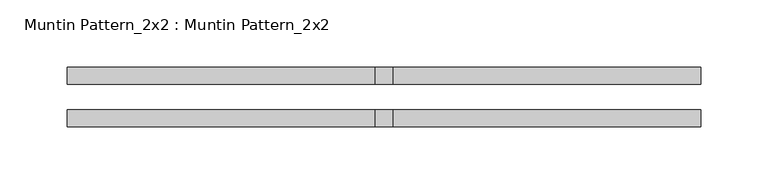
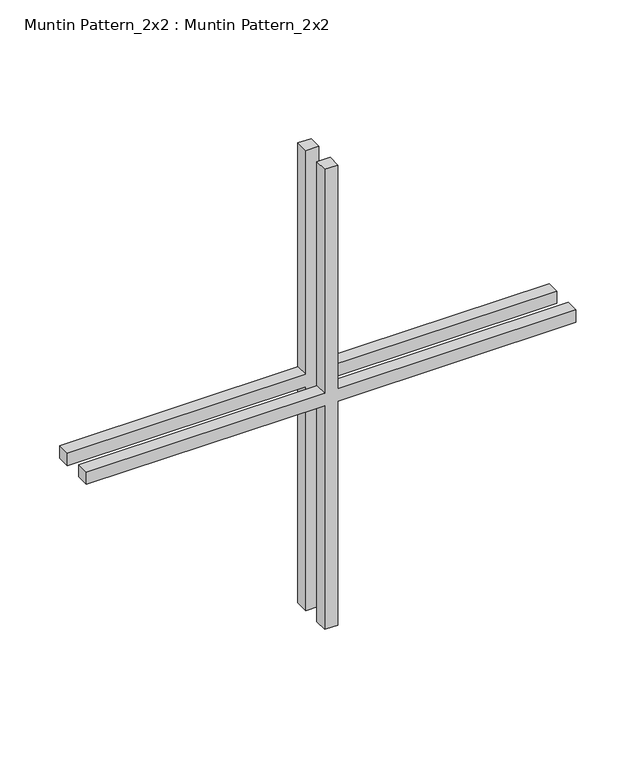
"""IFC4 building model written with IfcOpenShell, lengths in millimetres: proxy geometry, Muntin Pattern_2x2 : Muntin Pattern_2x2."""

from ifc_helpers import new_model, si_unit, frame, origin, place, context, project, spatial, polyline, outline, extrude, source, transform, mapped, element, save


def muntin_pattern_2x2_muntin_pattern_2x2_7d820091(model_context):
    return source(origin(), model_context, "Body", "SweptSolid", [
        extrude(outline(polyline([(241.3, -6.35), (241.3, -236.5375), (228.6, -236.5375), (228.6, -6.35), (0.0, -6.35), (0.0, 6.35), (228.6, 6.35), (228.6, 236.5375), (241.3, 236.5375), (241.3, 6.35), (469.9, 6.35), (469.9, -6.35), (241.3, -6.35)])), frame((0.0, 9.525, 0.0), z_axis=(0.0, 1.0, 0.0), x_axis=(0.0, 0.0, 1.0)), (0.0, 0.0, 1.0), 12.7),
        extrude(outline(polyline([(241.3, -6.35), (241.3, -236.5375), (228.6, -236.5375), (228.6, -6.35), (0.0, -6.35), (0.0, 6.35), (228.6, 6.35), (228.6, 236.5375), (241.3, 236.5375), (241.3, 6.35), (469.9, 6.35), (469.9, -6.35), (241.3, -6.35)])), frame((0.0, -22.225, 0.0), z_axis=(0.0, 1.0, 0.0), x_axis=(0.0, 0.0, 1.0)), (0.0, 0.0, 1.0), 12.7),
    ])


if __name__ == "__main__":
    model = new_model("IFC4")
    model_context = context("Model", 3, world=origin())
    ifc_project = project(units=[si_unit("LENGTHUNIT", "METRE", prefix="MILLI")], contexts=[model_context])
    site = spatial("IfcSite", under=ifc_project)
    building = spatial("IfcBuilding", under=site)
    placement = place(None, origin())
    muntin_pattern_2x2_muntin_pattern_2x2_shape = muntin_pattern_2x2_muntin_pattern_2x2_7d820091(model_context)
    element("IfcBuildingElementProxy", 1, Name="Muntin Pattern_2x2 : Muntin Pattern_2x2", ObjectType="Muntin Pattern_2x2 : Muntin Pattern_2x2", at=placement, inside=building, context=model_context, shape_type="MappedRepresentation", body=[
        mapped(muntin_pattern_2x2_muntin_pattern_2x2_shape, transform((0.0, 0.0, 0.0), x_axis=(1.0, 0.0, 0.0), y_axis=(0.0, 1.0, 0.0), z_axis=(0.0, 0.0, 1.0))),
    ])
    save(model, "model.ifc")

# Revit data of these elements
# Type "Muntin Pattern_2x2 : Muntin Pattern_2x2"
#   Width [instance default] = 4' - 0"
#   Thickness = 0' - 0 1/2"
#   Height [instance default] = 4' - 0"
#   Distance = 0' - 0 3/4"
#   Interior Material [instance default] = none
#   Exterior Material [instance default] = none
#   Default Elevation = 0
# Element 1 (IfcBuildingElementProxy, "Muntin Pattern_2x2 : Muntin Pattern_2x2")
#   Width = 1' - 6 5/8"
#   Height = 1' - 6 1/2"
#   Interior Material = Wood - Stained
#   Exterior Material = Clad - White
#   Materials on its faces: "Clad - White", "Wood - Stained"
# Materials
#   "Clad - White": class "Wood", colour RGB 242 242 238, transparency 0, Cost = 0
#   "Wood - Stained": class "Wood", colour RGB 224 178 126, transparency 0, Cost = 0
